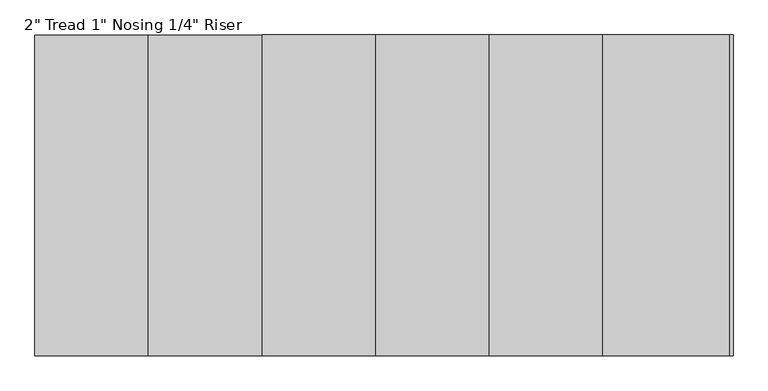
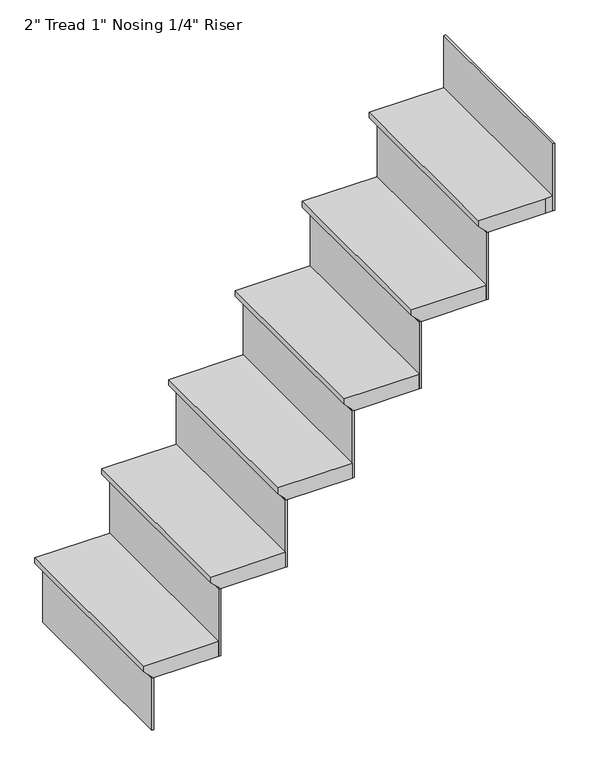
"""IFC4 building model written with IfcOpenShell, lengths in millimetres: stair flight geometry."""

from ifc_helpers import new_model, si_unit, origin, place, context, project, spatial, faceted_brep, source, transform, mapped, element, save


def stair_flight_1bfa81ce(model_context):
    return source(origin(), model_context, "Body", "Brep", [
        faceted_brep([(-4591.3634065, 3724.7702159, 6610.35), (-4591.3634065, 3724.7702159, 6629.4), (-4591.3634065, 4334.3702159, 6629.4), (-4591.3634065, 4334.3702159, 6610.35), (-4565.9634065, 3724.7702159, 6584.95), (-4565.9634065, 4334.3702159, 6584.95), (-4350.0634065, 3724.7702159, 6629.4), (-4350.0634065, 4334.3702159, 6629.4), (-4565.9634065, 4334.3702159, 6578.6), (-4350.0634065, 4334.3702159, 6578.6), (-4350.0634065, 3724.7702159, 6578.6), (-4565.9634065, 3724.7702159, 6578.6)], [[[0, 1, 2, 3]], [[4, 0, 3, 5]], [[2, 1, 6, 7]], [[8, 9, 10, 11]], [[2, 7, 9, 8, 5, 3]], [[8, 11, 4, 5]], [[6, 1, 0, 4, 11, 10]], [[7, 6, 10, 9]]]),
        faceted_brep([(-4565.9634065, 3724.7702159, 6578.6), (-4565.9634065, 3724.7702159, 6400.8), (-4559.6134065, 3724.7702159, 6400.8), (-4559.6134065, 3724.7702159, 6578.6), (-4565.9634065, 4334.3702159, 6578.6), (-4559.6134065, 4334.3702159, 6578.6), (-4559.6134065, 4334.3702159, 6400.8), (-4565.9634065, 4334.3702159, 6400.8)], [[[0, 1, 2, 3]], [[4, 5, 6, 7]], [[1, 0, 4, 7]], [[2, 1, 7, 6]], [[3, 2, 6, 5]], [[0, 3, 5, 4]]]),
        faceted_brep([(-3270.5634065, 3724.7702159, 7950.2), (-3270.5634065, 3724.7702159, 7721.6), (-3264.2134065, 3724.7702159, 7721.6), (-3264.2134065, 3724.7702159, 7950.2), (-3270.5634065, 4334.3702159, 7950.2), (-3264.2134065, 4334.3702159, 7950.2), (-3264.2134065, 4334.3702159, 7721.6), (-3270.5634065, 4334.3702159, 7721.6)], [[[0, 1, 2, 3]], [[4, 5, 6, 7]], [[1, 0, 4, 7]], [[2, 1, 7, 6]], [[3, 2, 6, 5]], [[0, 3, 5, 4]]]),
        faceted_brep([(-4350.0634065, 3724.7702159, 6807.2), (-4350.0634065, 3724.7702159, 6578.6), (-4343.7134065, 3724.7702159, 6578.6), (-4343.7134065, 3724.7702159, 6807.2), (-4350.0634065, 4334.3702159, 6807.2), (-4343.7134065, 4334.3702159, 6807.2), (-4343.7134065, 4334.3702159, 6578.6), (-4350.0634065, 4334.3702159, 6578.6)], [[[0, 1, 2, 3]], [[4, 5, 6, 7]], [[1, 0, 4, 7]], [[2, 1, 7, 6]], [[3, 2, 6, 5]], [[0, 3, 5, 4]]]),
        faceted_brep([(-4375.4634065, 4334.3702159, 6858.0), (-4375.4634065, 3724.7702159, 6858.0), (-4134.1634065, 3724.7702159, 6858.0), (-4134.1634065, 4334.3702159, 6858.0), (-4350.0634065, 4334.3702159, 6807.2), (-4134.1634065, 4334.3702159, 6807.2), (-4134.1634065, 3724.7702159, 6807.2), (-4350.0634065, 3724.7702159, 6807.2), (-4350.0634065, 4334.3702159, 6813.55), (-4375.4634065, 4334.3702159, 6838.95), (-4350.0634065, 3724.7702159, 6813.55), (-4375.4634065, 3724.7702159, 6838.95)], [[[0, 1, 2, 3]], [[4, 5, 6, 7]], [[0, 3, 5, 4, 8, 9]], [[4, 7, 10, 8]], [[2, 1, 11, 10, 7, 6]], [[3, 2, 6, 5]], [[11, 1, 0, 9]], [[10, 11, 9, 8]]]),
        faceted_brep([(-4134.1634065, 3724.7702159, 7035.8), (-4134.1634065, 3724.7702159, 6807.2), (-4127.8134065, 3724.7702159, 6807.2), (-4127.8134065, 3724.7702159, 7035.8), (-4134.1634065, 4334.3702159, 7035.8), (-4127.8134065, 4334.3702159, 7035.8), (-4127.8134065, 4334.3702159, 6807.2), (-4134.1634065, 4334.3702159, 6807.2)], [[[0, 1, 2, 3]], [[4, 5, 6, 7]], [[1, 0, 4, 7]], [[2, 1, 7, 6]], [[3, 2, 6, 5]], [[0, 3, 5, 4]]]),
        faceted_brep([(-4159.5634065, 4334.3702159, 7086.6), (-4159.5634065, 3724.7702159, 7086.6), (-3918.2634065, 3724.7702159, 7086.6), (-3918.2634065, 4334.3702159, 7086.6), (-4134.1634065, 4334.3702159, 7035.8), (-3918.2634065, 4334.3702159, 7035.8), (-3918.2634065, 3724.7702159, 7035.8), (-4134.1634065, 3724.7702159, 7035.8), (-4134.1634065, 4334.3702159, 7042.15), (-4159.5634065, 4334.3702159, 7067.55), (-4134.1634065, 3724.7702159, 7042.15), (-4159.5634065, 3724.7702159, 7067.55)], [[[0, 1, 2, 3]], [[4, 5, 6, 7]], [[0, 3, 5, 4, 8, 9]], [[4, 7, 10, 8]], [[2, 1, 11, 10, 7, 6]], [[3, 2, 6, 5]], [[11, 1, 0, 9]], [[10, 11, 9, 8]]]),
        faceted_brep([(-3918.2634065, 3724.7702159, 7264.4), (-3918.2634065, 3724.7702159, 7035.8), (-3911.9134065, 3724.7702159, 7035.8), (-3911.9134065, 3724.7702159, 7264.4), (-3918.2634065, 4334.3702159, 7264.4), (-3911.9134065, 4334.3702159, 7264.4), (-3911.9134065, 4334.3702159, 7035.8), (-3918.2634065, 4334.3702159, 7035.8)], [[[0, 1, 2, 3]], [[4, 5, 6, 7]], [[1, 0, 4, 7]], [[2, 1, 7, 6]], [[3, 2, 6, 5]], [[0, 3, 5, 4]]]),
        faceted_brep([(-3943.6634065, 4334.3702159, 7315.2), (-3943.6634065, 3724.7702159, 7315.2), (-3702.3634065, 3724.7702159, 7315.2), (-3702.3634065, 4334.3702159, 7315.2), (-3918.2634065, 4334.3702159, 7264.4), (-3702.3634065, 4334.3702159, 7264.4), (-3702.3634065, 3724.7702159, 7264.4), (-3918.2634065, 3724.7702159, 7264.4), (-3918.2634065, 4334.3702159, 7270.75), (-3943.6634065, 4334.3702159, 7296.15), (-3918.2634065, 3724.7702159, 7270.75), (-3943.6634065, 3724.7702159, 7296.15)], [[[0, 1, 2, 3]], [[4, 5, 6, 7]], [[0, 3, 5, 4, 8, 9]], [[4, 7, 10, 8]], [[2, 1, 11, 10, 7, 6]], [[3, 2, 6, 5]], [[11, 1, 0, 9]], [[10, 11, 9, 8]]]),
        faceted_brep([(-3702.3634065, 3724.7702159, 7493.0), (-3702.3634065, 3724.7702159, 7264.4), (-3696.0134065, 3724.7702159, 7264.4), (-3696.0134065, 3724.7702159, 7493.0), (-3702.3634065, 4334.3702159, 7493.0), (-3696.0134065, 4334.3702159, 7493.0), (-3696.0134065, 4334.3702159, 7264.4), (-3702.3634065, 4334.3702159, 7264.4)], [[[0, 1, 2, 3]], [[4, 5, 6, 7]], [[1, 0, 4, 7]], [[2, 1, 7, 6]], [[3, 2, 6, 5]], [[0, 3, 5, 4]]]),
        faceted_brep([(-3727.7634065, 4334.3702159, 7543.8), (-3727.7634065, 3724.7702159, 7543.8), (-3486.4634065, 3724.7702159, 7543.8), (-3486.4634065, 4334.3702159, 7543.8), (-3702.3634065, 4334.3702159, 7493.0), (-3486.4634065, 4334.3702159, 7493.0), (-3486.4634065, 3724.7702159, 7493.0), (-3702.3634065, 3724.7702159, 7493.0), (-3702.3634065, 4334.3702159, 7499.35), (-3727.7634065, 4334.3702159, 7524.75), (-3702.3634065, 3724.7702159, 7499.35), (-3727.7634065, 3724.7702159, 7524.75)], [[[0, 1, 2, 3]], [[4, 5, 6, 7]], [[0, 3, 5, 4, 8, 9]], [[4, 7, 10, 8]], [[2, 1, 11, 10, 7, 6]], [[3, 2, 6, 5]], [[11, 1, 0, 9]], [[10, 11, 9, 8]]]),
        faceted_brep([(-3486.4634065, 3724.7702159, 7721.6), (-3486.4634065, 3724.7702159, 7493.0), (-3480.1134065, 3724.7702159, 7493.0), (-3480.1134065, 3724.7702159, 7721.6), (-3486.4634065, 4334.3702159, 7721.6), (-3480.1134065, 4334.3702159, 7721.6), (-3480.1134065, 4334.3702159, 7493.0), (-3486.4634065, 4334.3702159, 7493.0)], [[[0, 1, 2, 3]], [[4, 5, 6, 7]], [[1, 0, 4, 7]], [[2, 1, 7, 6]], [[3, 2, 6, 5]], [[0, 3, 5, 4]]]),
        faceted_brep([(-3511.8634065, 4334.3702159, 7772.4), (-3511.8634065, 3724.7702159, 7772.4), (-3295.9634065, 3724.7702159, 7772.4), (-3270.5634065, 3724.7702159, 7772.4), (-3270.5634065, 4334.3702159, 7772.4), (-3486.4634065, 4334.3702159, 7721.6), (-3270.5634065, 4334.3702159, 7721.6), (-3270.5634065, 3724.7702159, 7721.6), (-3295.9634065, 3724.7702159, 7721.6), (-3486.4634065, 3724.7702159, 7721.6), (-3486.4634065, 4334.3702159, 7727.95), (-3511.8634065, 4334.3702159, 7753.35), (-3486.4634065, 3724.7702159, 7727.95), (-3511.8634065, 3724.7702159, 7753.35)], [[[0, 1, 2, 3, 4]], [[5, 6, 7, 8, 9]], [[0, 4, 6, 5, 10, 11]], [[5, 9, 12, 10]], [[2, 1, 13, 12, 9, 8]], [[3, 2, 8, 7]], [[4, 3, 7, 6]], [[13, 1, 0, 11]], [[12, 13, 11, 10]]]),
    ])


if __name__ == "__main__":
    model = new_model("IFC4")
    model_context = context("Model", 3, world=origin())
    ifc_project = project(units=[si_unit("LENGTHUNIT", "METRE", prefix="MILLI")], contexts=[model_context])
    site = spatial("IfcSite", under=ifc_project)
    building = spatial("IfcBuilding", under=site)
    placement = place(None, origin())
    stair_flight_shape = stair_flight_1bfa81ce(model_context)
    element("IfcStairFlight", 1, ObjectType="2\" Tread 1\" Nosing 1/4\" Riser", at=placement, inside=building, context=model_context, shape_type="MappedRepresentation", body=[
        mapped(stair_flight_shape, transform((0.0, 0.0, 0.0), x_axis=(1.0, 0.0, 0.0), y_axis=(0.0, 1.0, 0.0), z_axis=(0.0, 0.0, 1.0))),
    ])
    save(model, "model.ifc")
